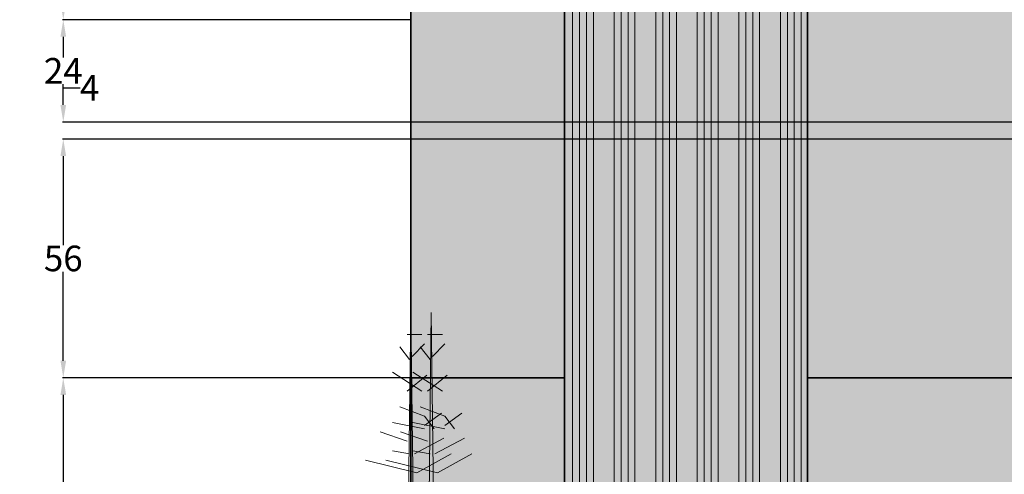
# Model space of a CAD drawing. Units: inches. Extents: x 221 to 874, y 171 to 738.
# Tile 3 of 11: x 221 to 452, y 348 to 455. Entities that reach past the tile are written whole.
import ezdxf

# ---------------------------------------------------------------- set-up
doc = ezdxf.new("R2010")
doc.units = ezdxf.units.IN
doc.header["$MEASUREMENT"] = 0
for name, color, linetype, lineweight in [('A-ANNO-DIMS', 2, 'Continuous', 18), ('A-ELEV', 7, 'Continuous', 35), ('A-ELEV-PATT', 8, 'Continuous', 13), ('L-PLNT', 3, 'Continuous', 13)]:
    doc.layers.add(name, color=color, linetype=linetype, lineweight=lineweight)
doc.styles.get("Standard").update_dxf_attribs({"font": 'arial.ttf'})
doc.dimstyles.get("Standard").update_dxf_attribs({"dimtxt": 6, "dimasz": 4, "dimexe": 0.18, "dimexo": 0.0625, "dimgap": 0.09, "dimtad": 0, "dimtih": 1, "dimtoh": 1, "dimdec": 0, "dimzin": 0, "dimdsep": 46, "dimlunit": 3, "dimtxsty": 'Standard', "dimcen": 0.09, "dimadec": 0, "dimazin": 0, "dimtfac": 1, "dimtdec": 0, "dimtofl": 0, "dimtmove": 0, "dimatfit": 3, "dimfxl": 1, "dimtolj": 1, "dimtzin": 0, "dimarcsym": 0})

# ---------------------------------------------------------------- blocks, each defined once
blk = doc.blocks.new('*D32')
at = {"layer": 'A-ANNO-DIMS', "color": 0, "lineweight": -2, "transparency": 16777216}
for p, q in [((313.02, 370.72), (231.36, 370.72)), ((231.54, 366.72), (231.54, 331.61)), ((231.54, 290.2), (231.54, 325.3)), ((313.02, 286.2), (231.36, 286.2))]:
    blk.add_line(p, q, dxfattribs=at)
at = {"layer": 'A-ANNO-DIMS', "color": 0, "transparency": 16777216}
for points in [[(230.88, 366.72), (232.21, 366.72), (231.54, 370.72)], [(230.88, 290.2), (232.21, 290.2), (231.54, 286.2)]]:
    blk.add_solid(points, dxfattribs=at)
at = {"layer": 'Defpoints', "color": 0, "transparency": 16777216}
for p in [(231.54, 370.72), (313.08, 370.72), (313.08, 286.2)]:
    blk.add_point(p, dxfattribs=at)
at = {"layer": 'A-ANNO-DIMS', "color": 0, "transparency": 16777216, "insert": (231.54, 328.46), "char_height": 6, "attachment_point": 5}
blk.add_mtext('\\A1;84.52', dxfattribs=at)
blk = doc.blocks.new('*D33')
at = {"layer": 'A-ANNO-DIMS', "color": 0, "lineweight": -2, "transparency": 16777216}
for p, q in [((469.02, 426.72), (231.36, 426.72)), ((231.54, 422.72), (231.54, 401.87)), ((231.54, 374.72), (231.54, 395.56)), ((313.02, 370.72), (231.36, 370.72))]:
    blk.add_line(p, q, dxfattribs=at)
at = {"layer": 'A-ANNO-DIMS', "color": 0, "transparency": 16777216}
for points in [[(230.88, 422.72), (232.21, 422.72), (231.54, 426.72)], [(230.88, 374.72), (232.21, 374.72), (231.54, 370.72)]]:
    blk.add_solid(points, dxfattribs=at)
at = {"layer": 'Defpoints', "color": 0, "transparency": 16777216}
for p in [(231.54, 426.72), (469.08, 426.72), (313.08, 370.72)]:
    blk.add_point(p, dxfattribs=at)
at = {"layer": 'A-ANNO-DIMS', "color": 0, "transparency": 16777216, "insert": (231.54, 398.72), "char_height": 6, "attachment_point": 5}
blk.add_mtext('\\A1;56', dxfattribs=at)
blk = doc.blocks.new('*D34')
at = {"layer": 'A-ANNO-DIMS', "color": 0, "lineweight": -2, "transparency": 16777216}
for p, q in [((231.54, 434.72), (231.54, 438.72)), ((231.54, 438.72), (235.54, 438.72)), ((469.02, 430.72), (231.36, 430.72)), ((469.02, 426.72), (231.36, 426.72)), ((231.54, 422.72), (231.54, 418.72))]:
    blk.add_line(p, q, dxfattribs=at)
at = {"layer": 'A-ANNO-DIMS', "color": 0, "transparency": 16777216}
for points in [[(230.88, 434.72), (232.21, 434.72), (231.54, 430.72)], [(230.88, 422.72), (232.21, 422.72), (231.54, 426.72)]]:
    blk.add_solid(points, dxfattribs=at)
at = {"layer": 'Defpoints', "color": 0, "transparency": 16777216}
for p in [(231.54, 430.72), (469.08, 430.72), (469.08, 426.72)]:
    blk.add_point(p, dxfattribs=at)
at = {"layer": 'A-ANNO-DIMS', "color": 0, "transparency": 16777216, "insert": (237.71, 438.72), "char_height": 6, "attachment_point": 5}
blk.add_mtext('\\A1;4', dxfattribs=at)
blk = doc.blocks.new('*D35')
at = {"layer": 'A-ANNO-DIMS', "color": 0, "lineweight": -2, "transparency": 16777216}
for p, q in [((313.02, 454.72), (231.36, 454.72)), ((231.54, 450.72), (231.54, 445.82)), ((231.54, 434.72), (231.54, 439.61)), ((469.02, 430.72), (231.36, 430.72))]:
    blk.add_line(p, q, dxfattribs=at)
at = {"layer": 'A-ANNO-DIMS', "color": 0, "transparency": 16777216}
for points in [[(230.88, 450.72), (232.21, 450.72), (231.54, 454.72)], [(230.88, 434.72), (232.21, 434.72), (231.54, 430.72)]]:
    blk.add_solid(points, dxfattribs=at)
at = {"layer": 'Defpoints', "color": 0, "transparency": 16777216}
for p in [(231.54, 454.72), (313.08, 454.72), (469.08, 430.72)]:
    blk.add_point(p, dxfattribs=at)
at = {"layer": 'A-ANNO-DIMS', "color": 0, "transparency": 16777216, "insert": (231.54, 442.72), "char_height": 6, "attachment_point": 5}
blk.add_mtext('\\A1;24', dxfattribs=at)
blk = doc.blocks.new('*D36')
at = {"layer": 'A-ANNO-DIMS', "color": 0, "lineweight": -2, "transparency": 16777216}
for p, q in [((313.02, 550.72), (231.36, 550.72)), ((231.54, 546.72), (231.54, 505.87)), ((231.54, 458.72), (231.54, 499.56)), ((313.02, 454.72), (231.36, 454.72))]:
    blk.add_line(p, q, dxfattribs=at)
at = {"layer": 'A-ANNO-DIMS', "color": 0, "transparency": 16777216}
for points in [[(230.88, 546.72), (232.21, 546.72), (231.54, 550.72)], [(230.88, 458.72), (232.21, 458.72), (231.54, 454.72)]]:
    blk.add_solid(points, dxfattribs=at)
at = {"layer": 'Defpoints', "color": 0, "transparency": 16777216}
for p in [(231.54, 550.72), (313.08, 550.72), (313.08, 454.72)]:
    blk.add_point(p, dxfattribs=at)
at = {"layer": 'A-ANNO-DIMS', "color": 0, "transparency": 16777216, "insert": (231.54, 502.72), "char_height": 6, "attachment_point": 5}
blk.add_mtext('\\A1;96', dxfattribs=at)

msp = doc.modelspace()

# ---------------------------------------------------------------- hatches: boundary and pattern name
at = {"layer": 'A-ELEV-PATT'}
h = msp.add_hatch(color=256, dxfattribs=at)
h.dxf.hatch_style = 1
h.paths.add_polyline_path([(349.0786, 286.1996), (313.0786, 286.1996), (313.0786, 232.7164), (349.0786, 232.7164)])
h.paths.add_polyline_path([(464.0786, 286.1996), (406.0786, 286.1996), (406.0786, 232.7164), (464.0786, 232.7164)])
h.paths.add_polyline_path([(541.0786, 286.1996), (493.0786, 286.1996), (493.0786, 232.7164), (541.0786, 232.7164)])
h.paths.add_polyline_path([(541.0786, 370.7164), (493.0786, 370.7164), (493.0786, 286.1996), (541.0786, 286.1996)])
h.paths.add_polyline_path([(464.0786, 370.7164), (406.0786, 370.7164), (406.0786, 286.1996), (464.0786, 286.1996)])
h.paths.add_polyline_path([(349.0786, 370.7164), (313.0786, 370.7164), (313.0786, 286.1996), (349.0786, 286.1996)])
h.paths.add_polyline_path([(349.0786, 454.7164), (313.0786, 454.7164), (313.0786, 370.7164), (349.0786, 370.7164)])
h.paths.add_polyline_path([(464.0786, 454.7164), (406.0786, 454.7164), (406.0786, 370.7164), (464.0786, 370.7164)])
h.paths.add_polyline_path([(541.0786, 418.7164), (541.0786, 454.7164), (493.0786, 454.7164), (493.0786, 370.7164), (541.0786, 370.7164)])
h.paths.add_polyline_path([(541.0786, 550.7164), (493.0786, 550.7164), (493.0786, 454.7164), (541.0786, 454.7164)])
h.paths.add_polyline_path([(464.0786, 550.7164), (406.0786, 550.7164), (406.0786, 454.7164), (464.0786, 454.7164)])
h.paths.add_polyline_path([(349.0786, 550.7164), (313.0786, 550.7164), (313.0786, 454.7164), (349.0786, 454.7164)])
h.paths.add_polyline_path([(349.0786, 586.7164), (313.0786, 586.7164), (313.0786, 550.7164), (349.0786, 550.7164)])
h.paths.add_polyline_path([(464.0786, 586.7164), (406.0786, 586.7164), (406.0786, 550.7164), (464.0786, 550.7164)])
h.paths.add_polyline_path([(541.0786, 574.7164), (541.0786, 586.7164), (493.0786, 586.7164), (493.0786, 550.7164), (541.0786, 550.7164)])
h.paths.add_polyline_path([(541.0786, 670.7164), (493.0786, 670.7164), (493.0786, 586.7164), (541.0786, 586.7164)])
h.paths.add_polyline_path([(464.0786, 670.7164), (406.0786, 670.7164), (406.0786, 586.7164), (464.0786, 586.7164)])
h.paths.add_polyline_path([(349.0786, 670.7164), (313.0786, 670.7164), (313.0786, 586.7164), (349.0786, 586.7164)])
h.paths.add_polyline_path([(406.0786, 706.7164), (313.0786, 706.7164), (313.0786, 670.7164), (349.0786, 670.7164), (406.0786, 670.7164)])
h.paths.add_polyline_path([(464.0786, 706.7164), (406.0786, 706.7164), (406.0786, 670.7164), (464.0786, 670.7164)])
h.paths.add_polyline_path([(541.0786, 706.7164), (493.0786, 706.7164), (493.0786, 688.7164), (493.0786, 670.7164), (541.0786, 670.7164)])
h.paths.add_polyline_path([(660.0786, 610.7164), (541.0786, 610.7164), (541.0786, 586.7164), (541.0786, 574.7164), (660.0786, 574.7164)])
h.paths.add_polyline_path([(781.0786, 610.7164), (660.0786, 610.7164), (660.0786, 574.7164), (769.0786, 574.7164), (781.0786, 574.7164)])
h.paths.add_polyline_path([(781.0786, 574.7164), (769.0786, 574.7164), (769.0786, 476.1199), (781.0786, 476.1199)])
h.paths.add_polyline_path([(781.0786, 476.1199), (769.0786, 476.1199), (769.0786, 457.7164), (781.0786, 457.7164)])
h.paths.add_polyline_path([(781.0786, 377.1023), (705.9097, 377.1023), (705.9097, 286.1996), (781.0786, 286.1996)])
h.paths.add_polyline_path([(741.9618, 338.8486), (756.9618, 338.8486), (756.9618, 329.8486), (741.9618, 329.8486)], flags=16)
h.paths.add_polyline_path([(648.9097, 377.1023), (598.0786, 377.1023), (598.0786, 286.1996), (648.9097, 286.1996)])
h.paths.add_polyline_path([(781.0786, 286.1996), (705.9097, 286.1996), (705.9097, 280.7164), (648.9097, 280.7164), (648.9097, 286.1996), (598.0786, 286.1996), (598.0786, 280.7164), (550.0786, 280.7164), (550.0786, 286.1996), (541.0786, 286.1996), (541.0786, 274.7164), (781.0786, 274.7164)])
h.paths.add_polyline_path([(660.0786, 562.7164), (546.3477, 562.7164), (546.3477, 457.7164), (660.0786, 457.7164)])
h = msp.add_hatch(color=256, dxfattribs=at)
h.paths.add_polyline_path([(406.0786, 670.7164), (349.0786, 670.7164), (349.0786, 454.7164), (406.0786, 454.7164)])
h.paths.add_polyline_path([(406.0786, 454.7164), (349.0786, 454.7164), (349.0786, 232.7164), (406.0786, 232.7164)])
h = msp.add_hatch(dxfattribs=at)
h.set_pattern_fill('ANSI34', color=256, scale=13, angle=45, style=0)
h.paths.add_polyline_path([(406.0786, 670.7164), (349.0786, 670.7164), (349.0786, 454.7164), (406.0786, 454.7164)])
h.paths.add_polyline_path([(406.0786, 454.7164), (349.0786, 454.7164), (349.0786, 232.7164), (406.0786, 232.7164)])

# ---------------------------------------------------------------- linework, layer by layer
at = {"layer": 'A-ELEV'}
for p, q in [((313.0786, 232.7164), (313.0786, 706.7164)), ((349.0786, 232.7164), (349.0786, 670.7164)), ((406.0786, 232.7164), (406.0786, 670.7164)), ((313.0786, 370.7164), (349.0786, 370.7164)), ((406.0786, 370.7164), (464.0786, 370.7164))]:
    msp.add_line(p, q, dxfattribs=at)
at = {"layer": 'L-PLNT'}
for p, q in [((313.0656, 386.0299), (310.9947, 220.2893)), ((313.0656, 386.0299), (315.358, 202.7164)), ((317.8656, 386.0299), (315.5752, 202.7164)), ((317.8656, 386.0299), (320.158, 202.7164)), ((312.2036, 380.8989), (315.6546, 380.8989)), ((317.0036, 380.8989), (320.4546, 380.8989)), ((310.4786, 377.9499), (312.7786, 375.0009)), ((313.3536, 375.7379), (316.2296, 378.6869)), ((315.2786, 377.9499), (317.5786, 375.0009)), ((318.1536, 375.7379), (321.0296, 378.6869)), ((308.7526, 372.0519), (315.6546, 367.6279)), ((313.5526, 372.0519), (320.4546, 367.6279)), ((312.2036, 367.6279), (316.8046, 371.3139)), ((317.0036, 367.6279), (321.6046, 371.3139)), ((310.4786, 363.9409), (316.2296, 361.7289)), ((315.2786, 363.9409), (321.0296, 361.7289)), ((316.2296, 359.5169), (320.2546, 362.4669)), ((316.2296, 361.7289), (318.5296, 358.7799)), ((321.0296, 359.5169), (325.0546, 362.4669)), ((321.0296, 361.7289), (323.3296, 358.7799)), ((312.2036, 355.8309), (305.8766, 358.0429)), ((308.7526, 360.2549), (316.2296, 358.7799)), ((317.0036, 355.8309), (310.6766, 358.0429)), ((313.5526, 360.2549), (321.0296, 358.7799)), ((313.9286, 352.8819), (320.8306, 356.5679)), ((318.7286, 352.8819), (325.6306, 356.5679)), ((308.7526, 353.6189), (312.7786, 352.8819)), ((313.5526, 353.6189), (317.5786, 352.8819)), ((314.5036, 348.4579), (302.4266, 351.4069)), ((319.3036, 348.4579), (307.2266, 351.4069)), ((322.5556, 352.8819), (314.5036, 348.4579)), ((327.3556, 352.8819), (319.3036, 348.4579))]:
    msp.add_line(p, q, dxfattribs=at)

# ---------------------------------------------------------------- dimensions: what is measured, and where the dimension line sits
at = {"layer": 'A-ANNO-DIMS'}
for base, p1, p2, override, picture, middle in [((231.5426, 550.7164), (313.0786, 454.7164), (313.0786, 550.7164), {"dimdec": 0, "dimlfac": 1, "dimrnd": 0, "dimzin": 0, "dimdsep": 46, "dimlunit": 2}, '*D36', (231.5426, 502.7164)), ((231.5426, 454.7164), (469.0786, 430.7164), (313.0786, 454.7164), {"dimdec": 0, "dimlfac": 1, "dimrnd": 0, "dimzin": 0, "dimdsep": 46, "dimlunit": 2}, '*D35', (231.5426, 442.7164)), ((231.5426, 430.7164), (469.0786, 426.7164), (469.0786, 430.7164), {"dimdec": 0, "dimlfac": 1, "dimrnd": 0, "dimzin": 0, "dimdsep": 46, "dimlunit": 2}, '*D34', (237.7077, 438.7164)), ((231.5426, 426.7164), (313.0786, 370.7164), (469.0786, 426.7164), {"dimdec": 0, "dimlfac": 1, "dimrnd": 0, "dimzin": 0, "dimdsep": 46, "dimlunit": 2}, '*D33', (231.5426, 398.7164)), ((231.5426, 370.7164), (313.0786, 286.1996), (313.0786, 370.7164), {"dimdec": 2, "dimlfac": 1, "dimrnd": 0, "dimzin": 0, "dimdsep": 46, "dimlunit": 2}, '*D32', (231.5426, 328.458))]:
    dim = msp.add_linear_dim(base=base, p1=p1, p2=p2, angle=90, dimstyle='Standard', override=override, dxfattribs=at)
    dim.commit()
    dim.dimension.update_dxf_attribs({"geometry": picture, "text_midpoint": middle})

doc.saveas('drawing.dxf')
